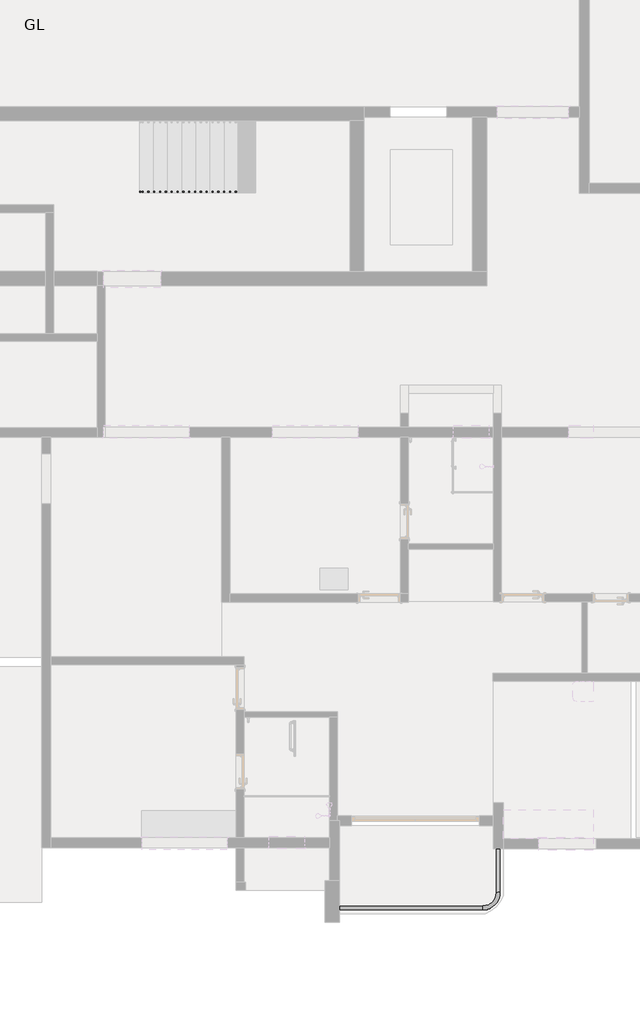
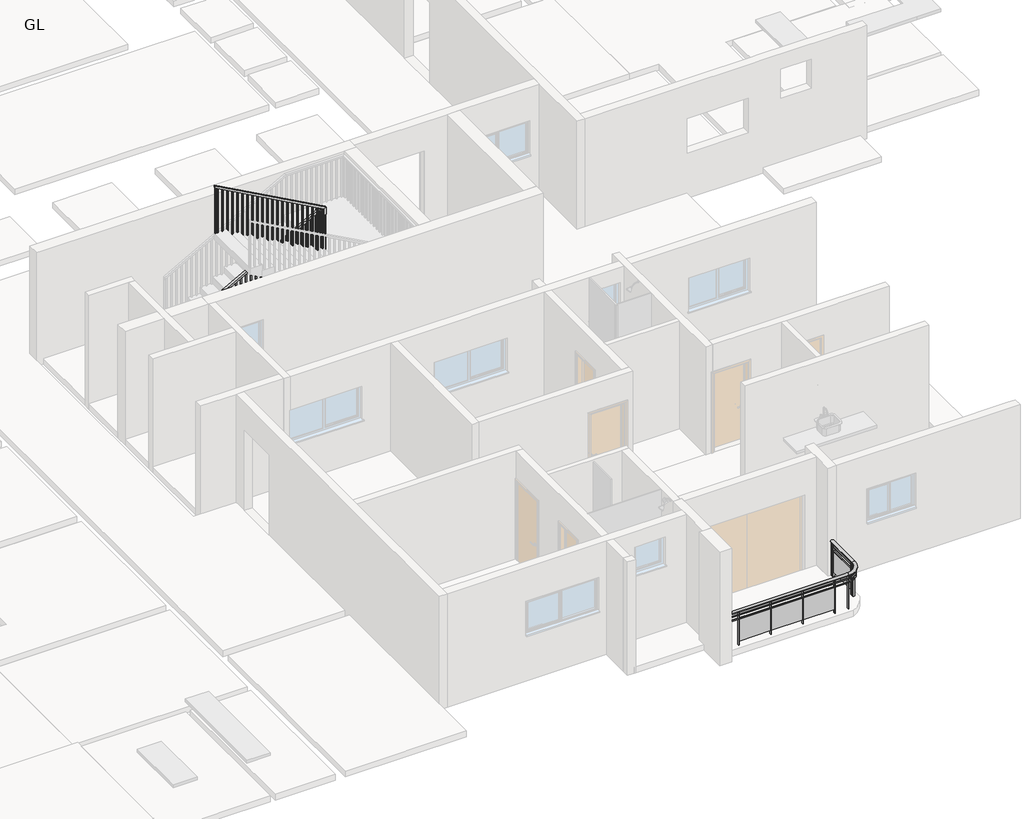
# One storey, part 9 of 14: 2 railings.
"""IFC4 building model written with IfcOpenShell, lengths in millimetres."""

from ifc_helpers import new_model, si_unit, point, frame, origin, place, context, project, spatial, polyline, circle_curve, ellipse_curve, trimmed, outline, extrude, faceted_brep, element, save
from ifc_brep_helpers import plane_surface, cylinder_surface, revolved_surface, extruded_surface, advanced_brep

model = new_model("IFC4")

# Units and contexts
model_context = context("Model", 3, world=origin())
ifc_project = project(units=[si_unit("LENGTHUNIT", "METRE", prefix="MILLI")], contexts=[model_context])

# Site, building, storey
site = spatial("IfcSite", under=ifc_project)
building = spatial("IfcBuilding", under=site)
storey = spatial("IfcBuildingStorey", under=building, Name="GL", Elevation=0.0)

# Railings
placement = place(None, origin())
element("IfcRailing", 1, ObjectType="1100mm", at=placement, inside=storey, context=model_context, shape_type="SolidModel", body=[
    faceted_brep([(-139.7980544, 71605.3236123, 1266.6666667), (-139.7980544, 71605.3236123, 1209.5692982), (-139.7980544, 71555.3236123, 1209.5692982), (-139.7980544, 71555.3236123, 1266.6666667), (2808.2019456, 71605.3236123, 2892.1987693), (2858.2019456, 71605.3236123, 2862.671484), (2858.2019456, 71555.3236123, 2862.671484), (2808.2019456, 71555.3236123, 2892.1987693), (2808.2019456, 71605.3236123, 2933.3333333), (2858.2019456, 71605.3236123, 2883.3333333), (2858.2019456, 71555.3236123, 2883.3333333), (2808.2019456, 71555.3236123, 2933.3333333), (2933.2019456, 71605.3236123, 2933.3333333), (2933.2019456, 71605.3236123, 2883.3333333), (2883.2019456, 71555.3236123, 2883.3333333), (2883.2019456, 71555.3236123, 2933.3333333), (2933.2019456, 71480.3236123, 2933.3333333), (2933.2019456, 71480.3236123, 2883.3333333), (2883.2019456, 71480.3236123, 2883.3333333), (2883.2019456, 71480.3236123, 2933.3333333), (2933.2019456, 71414.8236123, 2933.3333333), (2883.2019456, 71414.8236123, 2933.3333333), (2883.2019456, 71364.8236123, 2883.3333333), (2933.2019456, 71364.8236123, 2883.3333333)], [[[0, 1, 2, 3]], [[1, 0, 4, 5]], [[2, 1, 5, 6]], [[3, 2, 6, 7]], [[0, 3, 7, 4]], [[5, 4, 8, 9]], [[6, 5, 9, 10]], [[7, 6, 10, 11]], [[4, 7, 11, 8]], [[9, 8, 12, 13]], [[10, 9, 13, 14]], [[11, 10, 14, 15]], [[8, 11, 15, 12]], [[13, 12, 16, 17]], [[14, 13, 17, 18]], [[15, 14, 18, 19]], [[12, 15, 19, 16]], [[20, 21, 22, 23]], [[17, 16, 20, 23]], [[18, 17, 23, 22]], [[19, 18, 22, 21]], [[16, 19, 21, 20]]]),
    faceted_brep([(2933.2019456, 71414.8236123, 2933.3333333), (2933.2019456, 71364.8236123, 2883.3333333), (2883.2019456, 71364.8236123, 2883.3333333), (2883.2019456, 71414.8236123, 2933.3333333), (2933.2019456, 71414.8236123, 3072.2482242), (2883.2019456, 71414.8236123, 3042.7009883), (2883.2019456, 71364.8236123, 3042.7009883), (2933.2019456, 71364.8236123, 3072.2482242)], [[[0, 1, 2, 3]], [[4, 5, 6, 7]], [[1, 0, 4, 7]], [[2, 1, 7, 6]], [[3, 2, 6, 5]], [[0, 3, 5, 4]]]),
    faceted_brep([(2933.2019456, 71364.8236123, 3072.2482242), (2883.2019456, 71364.8236123, 3042.7009883), (2883.2019456, 71414.8236123, 3042.7009883), (2933.2019456, 71414.8236123, 3072.2482242), (158.6519456, 71364.8236123, 4600.0), (158.6519456, 71414.8236123, 4600.0), (158.6519456, 71414.8236123, 4542.9212405), (158.6519456, 71364.8236123, 4542.9212405)], [[[0, 1, 2, 3]], [[4, 5, 6, 7]], [[1, 0, 4, 7]], [[2, 1, 7, 6]], [[3, 2, 6, 5]], [[0, 3, 5, 4]]]),
    extrude(outline(polyline([(3333.3333333, 233.2019456), (4501.8717388, 233.2019456), (4515.6375006, 208.2019456), (3333.3333333, 208.2019456), (3333.3333333, 233.2019456)])), frame((0.0, 71377.3236123, 0.0), z_axis=(0.0, 1.0, 0.0), x_axis=(0.0, 0.0, 1.0)), (0.0, 0.0, 1.0), 25.0),
    extrude(outline(polyline([(3333.3333333, 358.2019456), (4433.0429298, 358.2019456), (4446.8086916, 333.2019456), (3333.3333333, 333.2019456), (3333.3333333, 358.2019456)])), frame((0.0, 71377.3236123, 0.0), z_axis=(0.0, 1.0, 0.0), x_axis=(0.0, 0.0, 1.0)), (0.0, 0.0, 1.0), 25.0),
    extrude(outline(polyline([(3166.6666667, 483.2019456), (4364.2141208, 483.2019456), (4377.9798826, 458.2019456), (3166.6666667, 458.2019456), (3166.6666667, 483.2019456)])), frame((0.0, 71377.3236123, 0.0), z_axis=(0.0, 1.0, 0.0), x_axis=(0.0, 0.0, 1.0)), (0.0, 0.0, 1.0), 25.0),
    extrude(outline(polyline([(3166.6666667, 608.2019456), (4295.3853118, 608.2019456), (4309.1510736, 583.2019456), (3166.6666667, 583.2019456), (3166.6666667, 608.2019456)])), frame((0.0, 71377.3236123, 0.0), z_axis=(0.0, 1.0, 0.0), x_axis=(0.0, 0.0, 1.0)), (0.0, 0.0, 1.0), 25.0),
    extrude(outline(polyline([(3166.6666667, 733.2019456), (4226.5565028, 733.2019456), (4240.3222646, 708.2019456), (3166.6666667, 708.2019456), (3166.6666667, 733.2019456)])), frame((0.0, 71377.3236123, 0.0), z_axis=(0.0, 1.0, 0.0), x_axis=(0.0, 0.0, 1.0)), (0.0, 0.0, 1.0), 25.0),
    extrude(outline(polyline([(3000.0, 858.2019456), (4157.7276938, 858.2019456), (4171.4934556, 833.2019456), (3000.0, 833.2019456), (3000.0, 858.2019456)])), frame((0.0, 71377.3236123, 0.0), z_axis=(0.0, 1.0, 0.0), x_axis=(0.0, 0.0, 1.0)), (0.0, 0.0, 1.0), 25.0),
    extrude(outline(polyline([(3000.0, 983.2019456), (4088.8988849, 983.2019456), (4102.6646467, 958.2019456), (3000.0, 958.2019456), (3000.0, 983.2019456)])), frame((0.0, 71377.3236123, 0.0), z_axis=(0.0, 1.0, 0.0), x_axis=(0.0, 0.0, 1.0)), (0.0, 0.0, 1.0), 25.0),
    extrude(outline(polyline([(2833.3333333, 1108.2019456), (4020.0700759, 1108.2019456), (4033.8358377, 1083.2019456), (2833.3333333, 1083.2019456), (2833.3333333, 1108.2019456)])), frame((0.0, 71377.3236123, 0.0), z_axis=(0.0, 1.0, 0.0), x_axis=(0.0, 0.0, 1.0)), (0.0, 0.0, 1.0), 25.0),
    extrude(outline(polyline([(2833.3333333, 1233.2019456), (3951.2412669, 1233.2019456), (3965.0070287, 1208.2019456), (2833.3333333, 1208.2019456), (2833.3333333, 1233.2019456)])), frame((0.0, 71377.3236123, 0.0), z_axis=(0.0, 1.0, 0.0), x_axis=(0.0, 0.0, 1.0)), (0.0, 0.0, 1.0), 25.0),
    extrude(outline(polyline([(2833.3333333, 1358.2019456), (3882.4124579, 1358.2019456), (3896.1782197, 1333.2019456), (2833.3333333, 1333.2019456), (2833.3333333, 1358.2019456)])), frame((0.0, 71377.3236123, 0.0), z_axis=(0.0, 1.0, 0.0), x_axis=(0.0, 0.0, 1.0)), (0.0, 0.0, 1.0), 25.0),
    extrude(outline(polyline([(2666.6666667, 1483.2019456), (3813.5836489, 1483.2019456), (3827.3494107, 1458.2019456), (2666.6666667, 1458.2019456), (2666.6666667, 1483.2019456)])), frame((0.0, 71377.3236123, 0.0), z_axis=(0.0, 1.0, 0.0), x_axis=(0.0, 0.0, 1.0)), (0.0, 0.0, 1.0), 25.0),
    extrude(outline(polyline([(2666.6666667, 1608.2019456), (3744.7548399, 1608.2019456), (3758.5206017, 1583.2019456), (2666.6666667, 1583.2019456), (2666.6666667, 1608.2019456)])), frame((0.0, 71377.3236123, 0.0), z_axis=(0.0, 1.0, 0.0), x_axis=(0.0, 0.0, 1.0)), (0.0, 0.0, 1.0), 25.0),
    extrude(outline(polyline([(2500.0, 1733.2019456), (3675.9260309, 1733.2019456), (3689.6917927, 1708.2019456), (2500.0, 1708.2019456), (2500.0, 1733.2019456)])), frame((0.0, 71377.3236123, 0.0), z_axis=(0.0, 1.0, 0.0), x_axis=(0.0, 0.0, 1.0)), (0.0, 0.0, 1.0), 25.0),
    extrude(outline(polyline([(2500.0, 1858.2019456), (3607.097222, 1858.2019456), (3620.8629837, 1833.2019456), (2500.0, 1833.2019456), (2500.0, 1858.2019456)])), frame((0.0, 71377.3236123, 0.0), z_axis=(0.0, 1.0, 0.0), x_axis=(0.0, 0.0, 1.0)), (0.0, 0.0, 1.0), 25.0),
    extrude(outline(polyline([(2500.0, 1983.2019456), (3538.268413, 1983.2019456), (3552.0341748, 1958.2019456), (2500.0, 1958.2019456), (2500.0, 1983.2019456)])), frame((0.0, 71377.3236123, 0.0), z_axis=(0.0, 1.0, 0.0), x_axis=(0.0, 0.0, 1.0)), (0.0, 0.0, 1.0), 25.0),
    extrude(outline(polyline([(2333.3333333, 2108.2019456), (3469.439604, 2108.2019456), (3483.2053658, 2083.2019456), (2333.3333333, 2083.2019456), (2333.3333333, 2108.2019456)])), frame((0.0, 71377.3236123, 0.0), z_axis=(0.0, 1.0, 0.0), x_axis=(0.0, 0.0, 1.0)), (0.0, 0.0, 1.0), 25.0),
    extrude(outline(polyline([(2333.3333333, 2233.2019456), (3400.610795, 2233.2019456), (3414.3765568, 2208.2019456), (2333.3333333, 2208.2019456), (2333.3333333, 2233.2019456)])), frame((0.0, 71377.3236123, 0.0), z_axis=(0.0, 1.0, 0.0), x_axis=(0.0, 0.0, 1.0)), (0.0, 0.0, 1.0), 25.0),
    extrude(outline(polyline([(2166.6666667, 2358.2019456), (3331.781986, 2358.2019456), (3345.5477478, 2333.2019456), (2166.6666667, 2333.2019456), (2166.6666667, 2358.2019456)])), frame((0.0, 71377.3236123, 0.0), z_axis=(0.0, 1.0, 0.0), x_axis=(0.0, 0.0, 1.0)), (0.0, 0.0, 1.0), 25.0),
    extrude(outline(polyline([(2166.6666667, 2483.2019456), (3262.953177, 2483.2019456), (3276.7189388, 2458.2019456), (2166.6666667, 2458.2019456), (2166.6666667, 2483.2019456)])), frame((0.0, 71377.3236123, 0.0), z_axis=(0.0, 1.0, 0.0), x_axis=(0.0, 0.0, 1.0)), (0.0, 0.0, 1.0), 25.0),
    extrude(outline(polyline([(2000.0, 2608.2019456), (3194.124368, 2608.2019456), (3207.8901298, 2583.2019456), (2000.0, 2583.2019456), (2000.0, 2608.2019456)])), frame((0.0, 71377.3236123, 0.0), z_axis=(0.0, 1.0, 0.0), x_axis=(0.0, 0.0, 1.0)), (0.0, 0.0, 1.0), 25.0),
    extrude(outline(polyline([(2000.0, 2733.2019456), (3125.295559, 2733.2019456), (3139.0613208, 2708.2019456), (2000.0, 2708.2019456), (2000.0, 2733.2019456)])), frame((0.0, 71377.3236123, 0.0), z_axis=(0.0, 1.0, 0.0), x_axis=(0.0, 0.0, 1.0)), (0.0, 0.0, 1.0), 25.0),
    extrude(outline(polyline([(2000.0, 2858.2019456), (3056.4667501, 2858.2019456), (3070.2325119, 2833.2019456), (2000.0, 2833.2019456), (2000.0, 2858.2019456)])), frame((0.0, 71377.3236123, 0.0), z_axis=(0.0, 1.0, 0.0), x_axis=(0.0, 0.0, 1.0)), (0.0, 0.0, 1.0), 25.0),
    extrude(outline(polyline([(2895.7019456, 71405.3236123), (2920.7019456, 71405.3236123), (2920.7019456, 71380.3236123), (2895.7019456, 71380.3236123), (2895.7019456, 71405.3236123)])), frame((0.0, 0.0, 1833.3333333), z_axis=(0.0, 0.0, 1.0), x_axis=(1.0, 0.0, 0.0)), (0.0, 0.0, 1.0), 1050.0),
    extrude(outline(polyline([(2895.7019456, 71530.3236123), (2920.7019456, 71530.3236123), (2920.7019456, 71505.3236123), (2895.7019456, 71505.3236123), (2895.7019456, 71530.3236123)])), frame((0.0, 0.0, 1833.3333333), z_axis=(0.0, 0.0, 1.0), x_axis=(1.0, 0.0, 0.0)), (0.0, 0.0, 1.0), 1050.0),
    extrude(outline(polyline([(2822.4191626, 2785.2019456), (1666.6666667, 2785.2019456), (1666.6666667, 2810.2019456), (2836.2042041, 2810.2019456), (2822.4191626, 2785.2019456)])), frame((0.0, 71567.8236123, 0.0), z_axis=(0.0, 1.0, 0.0), x_axis=(0.0, 0.0, 1.0)), (0.0, 0.0, 1.0), 25.0),
    extrude(outline(polyline([(2753.4939547, 2660.2019456), (1666.6666667, 2660.2019456), (1666.6666667, 2685.2019456), (2767.2789963, 2685.2019456), (2753.4939547, 2660.2019456)])), frame((0.0, 71567.8236123, 0.0), z_axis=(0.0, 1.0, 0.0), x_axis=(0.0, 0.0, 1.0)), (0.0, 0.0, 1.0), 25.0),
    extrude(outline(polyline([(2684.5687468, 2535.2019456), (1500.0, 2535.2019456), (1500.0, 2560.2019456), (2698.3537884, 2560.2019456), (2684.5687468, 2535.2019456)])), frame((0.0, 71567.8236123, 0.0), z_axis=(0.0, 1.0, 0.0), x_axis=(0.0, 0.0, 1.0)), (0.0, 0.0, 1.0), 25.0),
    extrude(outline(polyline([(2615.6435389, 2410.2019456), (1500.0, 2410.2019456), (1500.0, 2435.2019456), (2629.4285805, 2435.2019456), (2615.6435389, 2410.2019456)])), frame((0.0, 71567.8236123, 0.0), z_axis=(0.0, 1.0, 0.0), x_axis=(0.0, 0.0, 1.0)), (0.0, 0.0, 1.0), 25.0),
    extrude(outline(polyline([(2546.718331, 2285.2019456), (1500.0, 2285.2019456), (1500.0, 2310.2019456), (2560.5033726, 2310.2019456), (2546.718331, 2285.2019456)])), frame((0.0, 71567.8236123, 0.0), z_axis=(0.0, 1.0, 0.0), x_axis=(0.0, 0.0, 1.0)), (0.0, 0.0, 1.0), 25.0),
    extrude(outline(polyline([(2477.7931232, 2160.2019456), (1333.3333333, 2160.2019456), (1333.3333333, 2185.2019456), (2491.5781647, 2185.2019456), (2477.7931232, 2160.2019456)])), frame((0.0, 71567.8236123, 0.0), z_axis=(0.0, 1.0, 0.0), x_axis=(0.0, 0.0, 1.0)), (0.0, 0.0, 1.0), 25.0),
    extrude(outline(polyline([(2408.8679153, 2035.2019456), (1333.3333333, 2035.2019456), (1333.3333333, 2060.2019456), (2422.6529569, 2060.2019456), (2408.8679153, 2035.2019456)])), frame((0.0, 71567.8236123, 0.0), z_axis=(0.0, 1.0, 0.0), x_axis=(0.0, 0.0, 1.0)), (0.0, 0.0, 1.0), 25.0),
    extrude(outline(polyline([(2339.9427074, 1910.2019456), (1166.6666667, 1910.2019456), (1166.6666667, 1935.2019456), (2353.727749, 1935.2019456), (2339.9427074, 1910.2019456)])), frame((0.0, 71567.8236123, 0.0), z_axis=(0.0, 1.0, 0.0), x_axis=(0.0, 0.0, 1.0)), (0.0, 0.0, 1.0), 25.0),
    extrude(outline(polyline([(2271.0174995, 1785.2019456), (1166.6666667, 1785.2019456), (1166.6666667, 1810.2019456), (2284.8025411, 1810.2019456), (2271.0174995, 1785.2019456)])), frame((0.0, 71567.8236123, 0.0), z_axis=(0.0, 1.0, 0.0), x_axis=(0.0, 0.0, 1.0)), (0.0, 0.0, 1.0), 25.0),
    extrude(outline(polyline([(2202.0922917, 1660.2019456), (1000.0, 1660.2019456), (1000.0, 1685.2019456), (2215.8773332, 1685.2019456), (2202.0922917, 1660.2019456)])), frame((0.0, 71567.8236123, 0.0), z_axis=(0.0, 1.0, 0.0), x_axis=(0.0, 0.0, 1.0)), (0.0, 0.0, 1.0), 25.0),
    extrude(outline(polyline([(2133.1670838, 1535.2019456), (1000.0, 1535.2019456), (1000.0, 1560.2019456), (2146.9521254, 1560.2019456), (2133.1670838, 1535.2019456)])), frame((0.0, 71567.8236123, 0.0), z_axis=(0.0, 1.0, 0.0), x_axis=(0.0, 0.0, 1.0)), (0.0, 0.0, 1.0), 25.0),
    extrude(outline(polyline([(2064.2418759, 1410.2019456), (1000.0, 1410.2019456), (1000.0, 1435.2019456), (2078.0269175, 1435.2019456), (2064.2418759, 1410.2019456)])), frame((0.0, 71567.8236123, 0.0), z_axis=(0.0, 1.0, 0.0), x_axis=(0.0, 0.0, 1.0)), (0.0, 0.0, 1.0), 25.0),
    extrude(outline(polyline([(1995.316668, 1285.2019456), (833.3333333, 1285.2019456), (833.3333333, 1310.2019456), (2009.1017096, 1310.2019456), (1995.316668, 1285.2019456)])), frame((0.0, 71567.8236123, 0.0), z_axis=(0.0, 1.0, 0.0), x_axis=(0.0, 0.0, 1.0)), (0.0, 0.0, 1.0), 25.0),
    extrude(outline(polyline([(1926.3914601, 1160.2019456), (833.3333333, 1160.2019456), (833.3333333, 1185.2019456), (1940.1765017, 1185.2019456), (1926.3914601, 1160.2019456)])), frame((0.0, 71567.8236123, 0.0), z_axis=(0.0, 1.0, 0.0), x_axis=(0.0, 0.0, 1.0)), (0.0, 0.0, 1.0), 25.0),
    extrude(outline(polyline([(1857.4662523, 1035.2019456), (666.6666667, 1035.2019456), (666.6666667, 1060.2019456), (1871.2512938, 1060.2019456), (1857.4662523, 1035.2019456)])), frame((0.0, 71567.8236123, 0.0), z_axis=(0.0, 1.0, 0.0), x_axis=(0.0, 0.0, 1.0)), (0.0, 0.0, 1.0), 25.0),
    extrude(outline(polyline([(1788.5410444, 910.2019456), (666.6666667, 910.2019456), (666.6666667, 935.2019456), (1802.326086, 935.2019456), (1788.5410444, 910.2019456)])), frame((0.0, 71567.8236123, 0.0), z_axis=(0.0, 1.0, 0.0), x_axis=(0.0, 0.0, 1.0)), (0.0, 0.0, 1.0), 25.0),
    extrude(outline(polyline([(1719.6158365, 785.2019456), (666.6666667, 785.2019456), (666.6666667, 810.2019456), (1733.4008781, 810.2019456), (1719.6158365, 785.2019456)])), frame((0.0, 71567.8236123, 0.0), z_axis=(0.0, 1.0, 0.0), x_axis=(0.0, 0.0, 1.0)), (0.0, 0.0, 1.0), 25.0),
    extrude(outline(polyline([(1650.6906286, 660.2019456), (500.0, 660.2019456), (500.0, 685.2019456), (1664.4756702, 685.2019456), (1650.6906286, 660.2019456)])), frame((0.0, 71567.8236123, 0.0), z_axis=(0.0, 1.0, 0.0), x_axis=(0.0, 0.0, 1.0)), (0.0, 0.0, 1.0), 25.0),
    extrude(outline(polyline([(1581.7654208, 535.2019456), (500.0, 535.2019456), (500.0, 560.2019456), (1595.5504623, 560.2019456), (1581.7654208, 535.2019456)])), frame((0.0, 71567.8236123, 0.0), z_axis=(0.0, 1.0, 0.0), x_axis=(0.0, 0.0, 1.0)), (0.0, 0.0, 1.0), 25.0),
    extrude(outline(polyline([(1512.8402129, 410.2019456), (333.3333333, 410.2019456), (333.3333333, 435.2019456), (1526.6252544, 435.2019456), (1512.8402129, 410.2019456)])), frame((0.0, 71567.8236123, 0.0), z_axis=(0.0, 1.0, 0.0), x_axis=(0.0, 0.0, 1.0)), (0.0, 0.0, 1.0), 25.0),
    extrude(outline(polyline([(1443.915005, 285.2019456), (333.3333333, 285.2019456), (333.3333333, 310.2019456), (1457.7000466, 310.2019456), (1443.915005, 285.2019456)])), frame((0.0, 71567.8236123, 0.0), z_axis=(0.0, 1.0, 0.0), x_axis=(0.0, 0.0, 1.0)), (0.0, 0.0, 1.0), 25.0),
    extrude(outline(polyline([(1374.9897971, 160.2019456), (333.3333333, 160.2019456), (333.3333333, 185.2019456), (1388.7748387, 185.2019456), (1374.9897971, 160.2019456)])), frame((0.0, 71567.8236123, 0.0), z_axis=(0.0, 1.0, 0.0), x_axis=(0.0, 0.0, 1.0)), (0.0, 0.0, 1.0), 25.0),
    extrude(outline(polyline([(1306.0645892, 35.2019456), (166.6666667, 35.2019456), (166.6666667, 60.2019456), (1319.8496308, 60.2019456), (1306.0645892, 35.2019456)])), frame((0.0, 71567.8236123, 0.0), z_axis=(0.0, 1.0, 0.0), x_axis=(0.0, 0.0, 1.0)), (0.0, 0.0, 1.0), 25.0),
    extrude(outline(polyline([(1237.1393814, -89.7980544), (166.6666667, -89.7980544), (166.6666667, -64.7980544), (1250.9244229, -64.7980544), (1237.1393814, -89.7980544)])), frame((0.0, 71567.8236123, 0.0), z_axis=(0.0, 1.0, 0.0), x_axis=(0.0, 0.0, 1.0)), (0.0, 0.0, 1.0), 25.0),
    extrude(outline(polyline([(2895.7019456, 71402.3236123), (2920.7019456, 71402.3236123), (2920.7019456, 71377.3236123), (2895.7019456, 71377.3236123), (2895.7019456, 71402.3236123)])), frame((0.0, 0.0, 1833.3333333), z_axis=(0.0, 0.0, 1.0), x_axis=(1.0, 0.0, 0.0)), (0.0, 0.0, 1.0), 1050.0),
    extrude(outline(polyline([(2895.7019456, 71567.8236123), (2895.7019456, 71592.8236123), (2920.7019456, 71592.8236123), (2920.7019456, 71567.8236123), (2895.7019456, 71567.8236123)])), frame((0.0, 0.0, 1833.3333333), z_axis=(0.0, 0.0, 1.0), x_axis=(1.0, 0.0, 0.0)), (0.0, 0.0, 1.0), 1050.0),
    extrude(outline(polyline([(3333.3333333, 183.6519456), (4529.1554787, 183.6519456), (4542.9212405, 158.6519456), (3333.3333333, 158.6519456), (3333.3333333, 183.6519456)])), frame((0.0, 71377.3236123, 0.0), z_axis=(0.0, 1.0, 0.0), x_axis=(0.0, 0.0, 1.0)), (0.0, 0.0, 1.0), 25.0),
    extrude(outline(polyline([(1209.5692982, -139.7980544), (166.6666667, -139.7980544), (166.6666667, -114.7980544), (1223.3543398, -114.7980544), (1209.5692982, -139.7980544)])), frame((0.0, 71567.8236123, 0.0), z_axis=(0.0, 1.0, 0.0), x_axis=(0.0, 0.0, 1.0)), (0.0, 0.0, 1.0), 25.0),
])
element("IfcRailing", 2, ObjectType="Glass_Panel-Bottom_Fill", at=placement, inside=storey, context=model_context, shape_type="SolidModel", body=[
    advanced_brep(
    [(4143.1833567, 56258.2187256, 1049.9616), (4143.1833567, 56178.2187256, 1049.9616), (7216.5833567, 56258.2187256, 1049.9616), (7216.5833567, 56178.2187256, 1049.9616), (7593.7425916, 56555.3779605, 1049.9616), (7513.7425916, 56555.3779605, 1049.9616), (7513.7425916, 57494.2833045, 1049.9616), (7593.7425916, 57494.2833045, 1049.9616)],
    [
        (0, 1, ellipse_curve(frame((4143.1833567, 56218.2187256, 1049.9616), z_axis=(-1.0, 0.0, 0.0), x_axis=(0.0, -1.0, 0.0)), 40.0, 30.0)),
        (1, 0, ellipse_curve(frame((4143.1833567, 56218.2187256, 1049.9616), z_axis=(-1.0, 0.0, 0.0), x_axis=(0.0, -1.0, 0.0)), 40.0, 30.0)),
        (0, 2),
        (2, 3, ellipse_curve(frame((7216.5833567, 56218.2187256, 1049.9616), z_axis=(-1.0, 0.0, 0.0), x_axis=(0.0, -1.0, 0.0)), 40.0, 30.0)),
        (3, 1),
        (3, 2, ellipse_curve(frame((7216.5833567, 56218.2187256, 1049.9616), z_axis=(-1.0, 0.0, 0.0), x_axis=(0.0, -1.0, 0.0)), 40.0, 30.0)),
        (4, 3, circle_curve(frame((7216.5833567, 56555.3779605, 1049.9616), z_axis=(0.0, 0.0, -1.0), x_axis=(0.0, -1.0, 0.0)), 377.1592348)),
        (2, 5, circle_curve(frame((7216.5833567, 56555.3779605, 1049.9616), z_axis=(0.0, 0.0, 1.0), x_axis=(0.0, -1.0, 0.0)), 297.1592348)),
        (5, 4, ellipse_curve(frame((7553.7425916, 56555.3779605, 1049.9616), z_axis=(0.0, -1.0, 0.0), x_axis=(1.0, 0.0, 0.0)), 40.0, 30.0)),
        (4, 5, ellipse_curve(frame((7553.7425916, 56555.3779605, 1049.9616), z_axis=(0.0, -1.0, 0.0), x_axis=(1.0, 0.0, 0.0)), 40.0, 30.0)),
        (6, 7, ellipse_curve(frame((7553.7425916, 57494.2833045, 1049.9616), z_axis=(0.0, 1.0, 0.0), x_axis=(1.0, 0.0, 0.0)), 40.0, 30.0)),
        (7, 6, ellipse_curve(frame((7553.7425916, 57494.2833045, 1049.9616), z_axis=(0.0, 1.0, 0.0), x_axis=(1.0, 0.0, 0.0)), 40.0, 30.0)),
        (5, 6),
        (7, 4),
    ],
    [
        plane_surface(frame((4143.1833567, 56218.2187256, 1049.9616), z_axis=(-1.0, 0.0, 0.0), x_axis=(0.0, 1.0, 0.0))),
        extruded_surface(trimmed(ellipse_curve(frame((7216.5833567, 56218.2187256, 1049.9616), z_axis=(-1.0, 0.0, 0.0), x_axis=(0.0, -1.0, 0.0)), 40.0, 30.0), [point((7216.5833567, 56258.2187256, 1049.9616))], [point((7216.5833567, 56178.2187256, 1049.9616))], True, "CARTESIAN"), (-3073.3999999999996, 0.0, 0.0), 3073.3999999999996),
        extruded_surface(trimmed(ellipse_curve(frame((7216.5833567, 56218.2187256, 1049.9616), z_axis=(-1.0, 0.0, 0.0), x_axis=(0.0, -1.0, 0.0)), 40.0, 30.0), [point((7216.5833567, 56178.2187256, 1049.9616))], [point((7216.5833567, 56258.2187256, 1049.9616))], True, "CARTESIAN"), (-3073.3999999999996, 0.0, 0.0), 3073.3999999999996),
        revolved_surface(trimmed(ellipse_curve(frame((7216.5833567, 56218.2187256, 1049.9616), z_axis=(-1.0, 0.0, 0.0), x_axis=(0.0, -1.0, 0.0)), 40.0, 30.0), [point((7216.5833567, 56258.2187256, 1049.9616))], [point((7216.5833567, 56178.2187256, 1049.9616))], True, "CARTESIAN"), (7216.5833567, 56555.3779605, 1049.9616), (0.0, 0.0, 1.0)),
        revolved_surface(trimmed(ellipse_curve(frame((7216.5833567, 56218.2187256, 1049.9616), z_axis=(-1.0, 0.0, 0.0), x_axis=(0.0, -1.0, 0.0)), 40.0, 30.0), [point((7216.5833567, 56178.2187256, 1049.9616))], [point((7216.5833567, 56258.2187256, 1049.9616))], True, "CARTESIAN"), (7216.5833567, 56555.3779605, 1049.9616), (0.0, 0.0, 1.0)),
        plane_surface(frame((7553.7425916, 57494.2833045, 1049.9616), z_axis=(0.0, 1.0, 0.0), x_axis=(0.0, 0.0, 1.0))),
        extruded_surface(trimmed(ellipse_curve(frame((7553.7425916, 57494.2833045, 1049.9616), z_axis=(0.0, -1.0, 0.0), x_axis=(1.0, 0.0, 0.0)), 40.0, 30.0), [point((7513.7425916, 57494.2833045, 1049.9616))], [point((7593.7425916, 57494.2833045, 1049.9616))], True, "CARTESIAN"), (0.0, -938.9053439999989, 0.0), 938.9053439999989),
        extruded_surface(trimmed(ellipse_curve(frame((7553.7425916, 57494.2833045, 1049.9616), z_axis=(0.0, -1.0, 0.0), x_axis=(1.0, 0.0, 0.0)), 40.0, 30.0), [point((7593.7425916, 57494.2833045, 1049.9616))], [point((7513.7425916, 57494.2833045, 1049.9616))], True, "CARTESIAN"), (0.0, -938.9053439999989, 0.0), 938.9053439999989),
    ],
    [
        (0, [[1, 2]]),
        (1, [[-1, 3, 4, 5]]),
        (2, [[-2, -5, 6, -3]]),
        (3, [[7, -4, 8, 9]]),
        (4, [[-8, -6, -7, 10]]),
        (5, [[11, 12]]),
        (6, [[-9, 13, -12, 14]]),
        (7, [[-10, -14, -11, -13]]),
    ],
),
    advanced_brep(
    [(4143.1833567, 56208.8279605, 949.9616), (4143.1833567, 56228.8279605, 949.9616), (4143.1833567, 56228.8279605, 929.9616), (4143.1833567, 56208.8279605, 929.9616), (7216.5833567, 56208.8279605, 949.9616), (7216.5833567, 56228.8279605, 949.9616), (7216.5833567, 56228.8279605, 929.9616), (7216.5833567, 56208.8279605, 929.9616), (7543.1333567, 56555.3779605, 949.9616), (7563.1333567, 56555.3779605, 949.9616), (7543.1333567, 56555.3779605, 929.9616), (7563.1333567, 56555.3779605, 929.9616), (7563.1333567, 57494.2833045, 949.9616), (7563.1333567, 57494.2833045, 929.9616), (7543.1333567, 57494.2833045, 929.9616), (7543.1333567, 57494.2833045, 949.9616)],
    [
        (0, 1),
        (1, 2),
        (2, 3),
        (3, 0),
        (0, 4),
        (4, 5),
        (5, 1),
        (5, 6),
        (6, 2),
        (6, 7),
        (7, 3),
        (7, 4),
        (8, 5, circle_curve(frame((7216.5833567, 56555.3779605, 949.9616), z_axis=(0.0, 0.0, -1.0), x_axis=(0.0, -1.0, 0.0)), 326.55)),
        (4, 9, circle_curve(frame((7216.5833567, 56555.3779605, 949.9616), z_axis=(0.0, 0.0, 1.0), x_axis=(0.0, -1.0, 0.0)), 346.55)),
        (9, 8),
        (10, 6, circle_curve(frame((7216.5833567, 56555.3779605, 929.9616), z_axis=(0.0, 0.0, -1.0), x_axis=(0.0, -1.0, 0.0)), 326.55)),
        (8, 10),
        (11, 7, circle_curve(frame((7216.5833567, 56555.3779605, 929.9616), z_axis=(0.0, 0.0, -1.0), x_axis=(0.0, -1.0, 0.0)), 346.55)),
        (10, 11),
        (11, 9),
        (12, 13),
        (13, 14),
        (14, 15),
        (15, 12),
        (9, 12),
        (15, 8),
        (14, 10),
        (13, 11),
    ],
    [
        plane_surface(frame((4143.1833567, 56218.8279605, 949.9616), z_axis=(-1.0, 0.0, 0.0), x_axis=(0.0, 1.0, 0.0))),
        plane_surface(frame((4143.1833567, 56208.8279605, 949.9616), z_axis=(0.0, 0.0, 1.0), x_axis=(1.0, 0.0, 0.0))),
        plane_surface(frame((4143.1833567, 56228.8279605, 949.9616), z_axis=(0.0, 1.0, 0.0), x_axis=(1.0, 0.0, 0.0))),
        plane_surface(frame((4143.1833567, 56228.8279605, 929.9616), z_axis=(0.0, 0.0, -1.0), x_axis=(1.0, 0.0, 0.0))),
        plane_surface(frame((4143.1833567, 56208.8279605, 929.9616), z_axis=(0.0, -1.0, 0.0), x_axis=(1.0, 0.0, 0.0))),
        plane_surface(frame((7216.5833567, 56555.3779605, 949.9616), z_axis=(0.0, 0.0, 1.0), x_axis=(0.0, -1.0, 0.0))),
        revolved_surface(polyline([(7216.5833567, 56228.8279605, 949.9616), (7216.5833567, 56228.8279605, 929.9616)]), (7216.5833567, 56555.3779605, 949.9616), (0.0, 0.0, 1.0)),
        plane_surface(frame((7216.5833567, 56555.3779605, 929.9616), z_axis=(0.0, 0.0, -1.0), x_axis=(0.0, -1.0, 0.0))),
        cylinder_surface(frame((7216.5833567, 56555.3779605, 949.9616), z_axis=(0.0, 0.0, 1.0), x_axis=(0.0, -1.0, 0.0)), 346.55),
        plane_surface(frame((7553.1333567, 57494.2833045, 949.9616), z_axis=(0.0, 1.0, 0.0), x_axis=(0.0, 0.0, 1.0))),
        plane_surface(frame((7563.1333567, 56555.3779605, 949.9616), z_axis=(0.0, 0.0, 1.0), x_axis=(0.0, 1.0, 0.0))),
        plane_surface(frame((7543.1333567, 56555.3779605, 949.9616), z_axis=(-1.0, 0.0, 0.0), x_axis=(0.0, 1.0, 0.0))),
        plane_surface(frame((7543.1333567, 56555.3779605, 929.9616), z_axis=(0.0, 0.0, -1.0), x_axis=(0.0, 1.0, 0.0))),
        plane_surface(frame((7563.1333567, 56555.3779605, 929.9616), z_axis=(1.0, 0.0, 0.0), x_axis=(0.0, 1.0, 0.0))),
    ],
    [
        (0, [[1, 2, 3, 4]]),
        (1, [[-1, 5, 6, 7]]),
        (2, [[-2, -7, 8, 9]]),
        (3, [[-3, -9, 10, 11]]),
        (4, [[-4, -11, 12, -5]]),
        (5, [[13, -6, 14, 15]]),
        (6, [[16, -8, -13, 17]]),
        (7, [[18, -10, -16, 19]]),
        (8, [[-14, -12, -18, 20]]),
        (9, [[21, 22, 23, 24]]),
        (10, [[-15, 25, -24, 26]]),
        (11, [[-17, -26, -23, 27]]),
        (12, [[-19, -27, -22, 28]]),
        (13, [[-20, -28, -21, -25]]),
    ],
),
    advanced_brep(
    [(4143.1833567, 56208.8279605, 849.9616), (4143.1833567, 56228.8279605, 849.9616), (4143.1833567, 56228.8279605, 829.9616), (4143.1833567, 56208.8279605, 829.9616), (7216.5833567, 56208.8279605, 849.9616), (7216.5833567, 56228.8279605, 849.9616), (7216.5833567, 56228.8279605, 829.9616), (7216.5833567, 56208.8279605, 829.9616), (7543.1333567, 56555.3779605, 849.9616), (7563.1333567, 56555.3779605, 849.9616), (7543.1333567, 56555.3779605, 829.9616), (7563.1333567, 56555.3779605, 829.9616), (7563.1333567, 57494.2833045, 849.9616), (7563.1333567, 57494.2833045, 829.9616), (7543.1333567, 57494.2833045, 829.9616), (7543.1333567, 57494.2833045, 849.9616)],
    [
        (0, 1),
        (1, 2),
        (2, 3),
        (3, 0),
        (0, 4),
        (4, 5),
        (5, 1),
        (5, 6),
        (6, 2),
        (6, 7),
        (7, 3),
        (7, 4),
        (8, 5, circle_curve(frame((7216.5833567, 56555.3779605, 849.9616), z_axis=(0.0, 0.0, -1.0), x_axis=(0.0, -1.0, 0.0)), 326.55)),
        (4, 9, circle_curve(frame((7216.5833567, 56555.3779605, 849.9616), z_axis=(0.0, 0.0, 1.0), x_axis=(0.0, -1.0, 0.0)), 346.55)),
        (9, 8),
        (10, 6, circle_curve(frame((7216.5833567, 56555.3779605, 829.9616), z_axis=(0.0, 0.0, -1.0), x_axis=(0.0, -1.0, 0.0)), 326.55)),
        (8, 10),
        (11, 7, circle_curve(frame((7216.5833567, 56555.3779605, 829.9616), z_axis=(0.0, 0.0, -1.0), x_axis=(0.0, -1.0, 0.0)), 346.55)),
        (10, 11),
        (11, 9),
        (12, 13),
        (13, 14),
        (14, 15),
        (15, 12),
        (9, 12),
        (15, 8),
        (14, 10),
        (13, 11),
    ],
    [
        plane_surface(frame((4143.1833567, 56218.8279605, 849.9616), z_axis=(-1.0, 0.0, 0.0), x_axis=(0.0, 1.0, 0.0))),
        plane_surface(frame((4143.1833567, 56208.8279605, 849.9616), z_axis=(0.0, 0.0, 1.0), x_axis=(1.0, 0.0, 0.0))),
        plane_surface(frame((4143.1833567, 56228.8279605, 849.9616), z_axis=(0.0, 1.0, 0.0), x_axis=(1.0, 0.0, 0.0))),
        plane_surface(frame((4143.1833567, 56228.8279605, 829.9616), z_axis=(0.0, 0.0, -1.0), x_axis=(1.0, 0.0, 0.0))),
        plane_surface(frame((4143.1833567, 56208.8279605, 829.9616), z_axis=(0.0, -1.0, 0.0), x_axis=(1.0, 0.0, 0.0))),
        plane_surface(frame((7216.5833567, 56555.3779605, 849.9616), z_axis=(0.0, 0.0, 1.0), x_axis=(0.0, -1.0, 0.0))),
        revolved_surface(polyline([(7216.5833567, 56228.8279605, 849.9616), (7216.5833567, 56228.8279605, 829.9616)]), (7216.5833567, 56555.3779605, 849.9616), (0.0, 0.0, 1.0)),
        plane_surface(frame((7216.5833567, 56555.3779605, 829.9616), z_axis=(0.0, 0.0, -1.0), x_axis=(0.0, -1.0, 0.0))),
        cylinder_surface(frame((7216.5833567, 56555.3779605, 849.9616), z_axis=(0.0, 0.0, 1.0), x_axis=(0.0, -1.0, 0.0)), 346.55),
        plane_surface(frame((7553.1333567, 57494.2833045, 849.9616), z_axis=(0.0, 1.0, 0.0), x_axis=(0.0, 0.0, 1.0))),
        plane_surface(frame((7563.1333567, 56555.3779605, 849.9616), z_axis=(0.0, 0.0, 1.0), x_axis=(0.0, 1.0, 0.0))),
        plane_surface(frame((7543.1333567, 56555.3779605, 849.9616), z_axis=(-1.0, 0.0, 0.0), x_axis=(0.0, 1.0, 0.0))),
        plane_surface(frame((7543.1333567, 56555.3779605, 829.9616), z_axis=(0.0, 0.0, -1.0), x_axis=(0.0, 1.0, 0.0))),
        plane_surface(frame((7563.1333567, 56555.3779605, 829.9616), z_axis=(1.0, 0.0, 0.0), x_axis=(0.0, 1.0, 0.0))),
    ],
    [
        (0, [[1, 2, 3, 4]]),
        (1, [[-1, 5, 6, 7]]),
        (2, [[-2, -7, 8, 9]]),
        (3, [[-3, -9, 10, 11]]),
        (4, [[-4, -11, 12, -5]]),
        (5, [[13, -6, 14, 15]]),
        (6, [[16, -8, -13, 17]]),
        (7, [[18, -10, -16, 19]]),
        (8, [[-14, -12, -18, 20]]),
        (9, [[21, 22, 23, 24]]),
        (10, [[-15, 25, -24, 26]]),
        (11, [[-17, -26, -23, 27]]),
        (12, [[-19, -27, -22, 28]]),
        (13, [[-20, -28, -21, -25]]),
    ],
),
    extrude(outline(polyline([(7528.1333567, 57418.8306325), (7528.1333567, 57430.8306325), (7578.1333567, 57430.8306325), (7578.1333567, 57418.8306325), (7528.1333567, 57418.8306325)])), frame((0.0, 0.0, 149.9616), z_axis=(0.0, 0.0, 1.0), x_axis=(1.0, 0.0, 0.0)), (0.0, 0.0, 1.0), 870.0),
    extrude(outline(polyline([(7554.8581668, 56624.8306325), (7554.8581668, 57424.8306325), (7559.8581668, 57424.8306325), (7559.8581668, 56624.8306325), (7554.8581668, 56624.8306325)])), frame((0.0, 0.0, 249.9616), z_axis=(0.0, 0.0, 1.0), x_axis=(1.0, 0.0, 0.0)), (0.0, 0.0, 1.0), 580.0),
    extrude(outline(polyline([(7528.1333567, 56618.8306325), (7528.1333567, 56630.8306325), (7578.1333567, 56630.8306325), (7578.1333567, 56618.8306325), (7528.1333567, 56618.8306325)])), frame((0.0, 0.0, 149.9616), z_axis=(0.0, 0.0, 1.0), x_axis=(1.0, 0.0, 0.0)), (0.0, 0.0, 1.0), 870.0),
    extrude(outline(polyline([(6873.8833567, 56243.8279605), (6885.8833567, 56243.8279605), (6885.8833567, 56193.8279605), (6873.8833567, 56193.8279605), (6873.8833567, 56243.8279605)])), frame((0.0, 0.0, 149.9616), z_axis=(0.0, 0.0, 1.0), x_axis=(1.0, 0.0, 0.0)), (0.0, 0.0, 1.0), 870.0),
    extrude(outline(polyline([(6079.8833567, 56217.1031504), (6879.8833567, 56217.1031504), (6879.8833567, 56212.1031504), (6079.8833567, 56212.1031504), (6079.8833567, 56217.1031504)])), frame((0.0, 0.0, 249.9616), z_axis=(0.0, 0.0, 1.0), x_axis=(1.0, 0.0, 0.0)), (0.0, 0.0, 1.0), 580.0),
    extrude(outline(polyline([(6073.8833567, 56243.8279605), (6085.8833567, 56243.8279605), (6085.8833567, 56193.8279605), (6073.8833567, 56193.8279605), (6073.8833567, 56243.8279605)])), frame((0.0, 0.0, 149.9616), z_axis=(0.0, 0.0, 1.0), x_axis=(1.0, 0.0, 0.0)), (0.0, 0.0, 1.0), 870.0),
    extrude(outline(polyline([(5279.8833567, 56217.1031504), (6079.8833567, 56217.1031504), (6079.8833567, 56212.1031504), (5279.8833567, 56212.1031504), (5279.8833567, 56217.1031504)])), frame((0.0, 0.0, 249.9616), z_axis=(0.0, 0.0, 1.0), x_axis=(1.0, 0.0, 0.0)), (0.0, 0.0, 1.0), 580.0),
    extrude(outline(polyline([(5273.8833567, 56243.8279605), (5285.8833567, 56243.8279605), (5285.8833567, 56193.8279605), (5273.8833567, 56193.8279605), (5273.8833567, 56243.8279605)])), frame((0.0, 0.0, 149.9616), z_axis=(0.0, 0.0, 1.0), x_axis=(1.0, 0.0, 0.0)), (0.0, 0.0, 1.0), 870.0),
    extrude(outline(polyline([(4479.8833567, 56217.1031504), (5279.8833567, 56217.1031504), (5279.8833567, 56212.1031504), (4479.8833567, 56212.1031504), (4479.8833567, 56217.1031504)])), frame((0.0, 0.0, 249.9616), z_axis=(0.0, 0.0, 1.0), x_axis=(1.0, 0.0, 0.0)), (0.0, 0.0, 1.0), 580.0),
    extrude(outline(polyline([(4473.8833567, 56243.8279605), (4485.8833567, 56243.8279605), (4485.8833567, 56193.8279605), (4473.8833567, 56193.8279605), (4473.8833567, 56243.8279605)])), frame((0.0, 0.0, 149.9616), z_axis=(0.0, 0.0, 1.0), x_axis=(1.0, 0.0, 0.0)), (0.0, 0.0, 1.0), 870.0),
    extrude(outline(polyline([(7528.1333567, 56549.3779605), (7528.1333567, 56561.3779605), (7578.1333567, 56561.3779605), (7578.1333567, 56549.3779605), (7528.1333567, 56549.3779605)])), frame((0.0, 0.0, 149.9616), z_axis=(0.0, 0.0, 1.0), x_axis=(1.0, 0.0, 0.0)), (0.0, 0.0, 1.0), 870.0),
    extrude(outline(polyline([(7210.5833567, 56243.8279605), (7222.5833567, 56243.8279605), (7222.5833567, 56193.8279605), (7210.5833567, 56193.8279605), (7210.5833567, 56243.8279605)])), frame((0.0, 0.0, 149.9616), z_axis=(0.0, 0.0, 1.0), x_axis=(1.0, 0.0, 0.0)), (0.0, 0.0, 1.0), 870.0),
    extrude(outline(polyline([(7528.1333567, 57486.2833045), (7528.1333567, 57498.2833045), (7578.1333567, 57498.2833045), (7578.1333567, 57486.2833045), (7528.1333567, 57486.2833045)])), frame((0.0, 0.0, 149.9616), z_axis=(0.0, 0.0, 1.0), x_axis=(1.0, 0.0, 0.0)), (0.0, 0.0, 1.0), 870.0),
    extrude(outline(polyline([(4139.1833567, 56243.8279605), (4151.1833567, 56243.8279605), (4151.1833567, 56193.8279605), (4139.1833567, 56193.8279605), (4139.1833567, 56243.8279605)])), frame((0.0, 0.0, 149.9616), z_axis=(0.0, 0.0, 1.0), x_axis=(1.0, 0.0, 0.0)), (0.0, 0.0, 1.0), 870.0),
])

save(model, "model.ifc")

# Revit data of these elements
# Type "1100mm"
#   built-in parameter 1008612 = 0.019685 (stored number, unit not read)
#   built-in parameter 1008611 = 0.019685 (stored number, unit not read)
#   built-in parameter 1008609 = 0.902231 (stored number, unit not read)
#   built-in parameter 1008604 = 0.19685 (stored number, unit not read)
#   built-in parameter 1008603 = 0.164042 (stored number, unit not read)
#   Railing Height = 3.608924 ft
#   built-in parameter 1008630 = 2
#   built-in parameter 1008610 = 2
#   built-in parameter 1008608 = 1
#   built-in parameter 1008618 = Baluster_Square : 25mm
# Type "Glass_Panel-Bottom_Fill"
#   built-in parameter 1008612 = 0.019685 (stored number, unit not read)
#   built-in parameter 1008611 = 0.019685 (stored number, unit not read)
#   built-in parameter 1008609 = 0.902231 (stored number, unit not read)
#   built-in parameter 1008604 = 0.19685 (stored number, unit not read)
#   built-in parameter 1008603 = 0.164042 (stored number, unit not read)
#   Railing Height = 2.952756 ft
#   built-in parameter 1008630 = 2
#   built-in parameter 1008610 = 2
# Element 1 (IfcRailing, "1100mm")
#   Phase Created = New Construction
# Element 2 (IfcRailing, "Glass_Panel-Bottom_Fill")
#   built-in parameter 1008621 = 0.492 (stored number, unit not read)
#   Phase Created = New Construction
#   Materials on its faces: "Metal - Stainless Steel,Polished", "Glass"
# Materials
#   "Metal - Stainless Steel,Polished": class "Metal", colour RGB 236 239 239, transparency 0, Cost = 0
#   "Glass": class "Glass", colour RGB 0 128 192, transparency 0.9, Description = "Soda Lime Glass", Cost = 0
